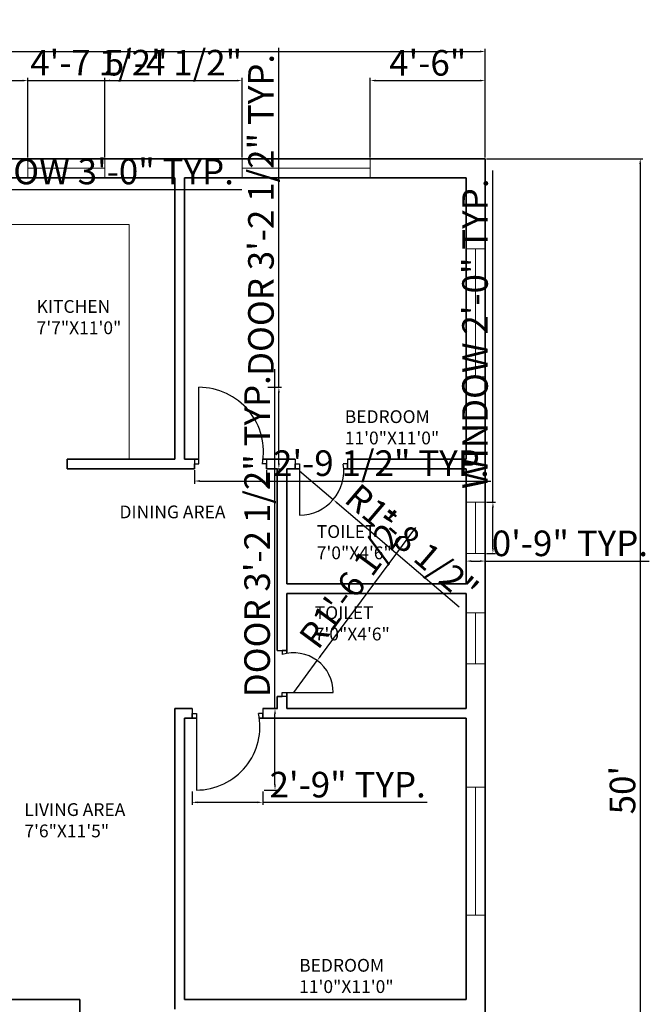
# Model space of a CAD drawing. Units: inches. Extents: x 2142 to 3604, y 1690 to 2981.
# Tile 3 of 9: x 2532 to 2827, y 2019 to 2481. Entities that reach past the tile are written whole.
import ezdxf

# ---------------------------------------------------------------- set-up
doc = ezdxf.new("R2010")
doc.units = ezdxf.units.IN
for name, color, linetype, lineweight in [('A-ANNO-DIMS', 2, 'Continuous', 18), ('A-AREA-IDEN', 7, 'Continuous', 18), ('A-DOOR', 4, 'Continuous', 25), ('A-FLOR-FIXT', 8, 'Continuous', 18), ('A-GLAZ', 4, 'Continuous', 18), ('A-WALL', 7, 'Continuous', 35)]:
    doc.layers.add(name, color=color, linetype=linetype, lineweight=lineweight)
doc.styles.get("Standard").update_dxf_attribs({"font": 'arial.ttf'})
doc.dimstyles.new('ISO-25', dxfattribs={"dimtxt": 12, "dimasz": 2.5, "dimexe": 1.25, "dimexo": 0.625, "dimtad": 1, "dimdec": 0, "dimlunit": 3, "dimtxsty": 'Standard', "dimcen": 2.5, "dimadec": 0, "dimazin": 0, "dimtfac": 1, "dimtdec": 0, "dimtmove": 0, "dimatfit": 3, "dimfxl": 1, "dimarcsym": 0})

# ---------------------------------------------------------------- blocks, each defined once
blk = doc.blocks.new('*D1')
at = {"layer": 'A-ANNO-DIMS', "color": 0, "lineweight": -2, "transparency": 16777216}
for p, q in [((2272.99, 2416.32), (2272.99, 2467.23)), ((2750.49, 2416.32), (2750.49, 2467.23)), ((2275.49, 2465.98), (2747.99, 2465.98))]:
    blk.add_line(p, q, dxfattribs=at)
at = {"layer": 'A-ANNO-DIMS', "color": 0, "transparency": 16777216}
for points in [[(2275.49, 2466.4), (2275.49, 2465.56), (2272.99, 2465.98)], [(2747.99, 2466.4), (2747.99, 2465.56), (2750.49, 2465.98)]]:
    blk.add_solid(points, dxfattribs=at)
at = {"layer": 'Defpoints', "color": 0, "transparency": 16777216}
for p in [(2750.49, 2465.98), (2272.99, 2415.7), (2750.49, 2415.7)]:
    blk.add_point(p, dxfattribs=at)
at = {"layer": 'A-ANNO-DIMS', "color": 0, "transparency": 16777216, "insert": (2511.74, 2472.73), "char_height": 12, "attachment_point": 5}
blk.add_mtext("40'", dxfattribs=at)
blk = doc.blocks.new('*D2')
at = {"layer": 'A-ANNO-DIMS', "color": 0, "lineweight": -2, "transparency": 16777216}
for p, q in [((2751.11, 2415.7), (2824.38, 2415.7)), ((2823.13, 2413.2), (2823.13, 1825.7)), ((2751.11, 1823.2), (2824.38, 1823.2))]:
    blk.add_line(p, q, dxfattribs=at)
at = {"layer": 'A-ANNO-DIMS', "color": 0, "transparency": 16777216}
for points in [[(2822.72, 2413.2), (2823.55, 2413.2), (2823.13, 2415.7)], [(2822.72, 1825.7), (2823.55, 1825.7), (2823.13, 1823.2)]]:
    blk.add_solid(points, dxfattribs=at)
at = {"layer": 'Defpoints', "color": 0, "transparency": 16777216}
for p in [(2750.49, 2415.7), (2750.49, 1823.2), (2823.13, 1823.2)]:
    blk.add_point(p, dxfattribs=at)
at = {"layer": 'A-ANNO-DIMS', "color": 0, "transparency": 16777216, "insert": (2816.38, 2119.45), "char_height": 12, "attachment_point": 5, "rotation": 90}
blk.add_mtext("50'", dxfattribs=at)
blk = doc.blocks.new('DOOR-BED-REAR-R')
for p, q in [((2, 2.25), (2, 38.25)), ((0, 4.5), (0, 0)), ((0, 0), (0, 2.25)), ((0, 2.25), (2, 2.25)), ((33.74, 2.25), (31.74, 2.25)), ((33.74, 4.5), (33.74, 0)), ((33.74, 0), (33.74, 2.25))]:
    blk.add_line(p, q)
blk.add_arc((2, 7.96), 30.29, 349.1278, 90)
blk = doc.blocks.new('DOOR-BATH-REAR-R')
for p, q in [((0, 26.25), (0, 21.75)), ((0, 21.75), (0, 24)), ((0, 24), (2, 24)), ((2, 24), (2, 0)), ((24.48, 24), (22.48, 24)), ((24.48, 26.25), (24.48, 21.75)), ((24.48, 21.75), (24.48, 24))]:
    blk.add_line(p, q)
blk.add_arc((2, 20.74), 20.74, 270, 9.0396)
blk = doc.blocks.new('DOOR-BATH-FRONT-R')
for p, q in [((0, 21.72), (4.5, 21.72)), ((4.5, 21.72), (2.25, 21.72)), ((2.25, 21.72), (2.25, 19.72)), ((4.5, 0), (0, 0)), ((0, 0), (2.25, 0)), ((2.25, 0), (2.25, 2)), ((2.25, 2), (26.25, 2))]:
    blk.add_line(p, q)
blk.add_arc((7.71, 2), 18.54, 0, 107.1246)
blk = doc.blocks.new('DOOR-BED-MID-R')
for p, q in [((0, 38.25), (0, 33.75)), ((33.13, 38.25), (33.13, 33.75)), ((0, 33.75), (0, 36)), ((0, 36), (2, 36)), ((2, 36), (2, 0)), ((33.13, 36), (31.13, 36)), ((33.13, 33.75), (33.13, 36))]:
    blk.add_line(p, q)
blk.add_arc((2, 29.79), 29.79, 270, 12.0368)
blk = doc.blocks.new('COUNTER-KITCHEN-R')
for p, q in [((0, 110.14), (69.54, 110.14)), ((69.54, 110.14), (69.54, 0))]:
    blk.add_line(p, q)
blk = doc.blocks.new('WINDOW-60')
for p, q in [((0, 60), (9, 60)), ((9, 60), (4.5, 60)), ((4.5, 60), (4.5, 0)), ((4.5, 0), (0, 0)), ((0, 0), (9, 0))]:
    blk.add_line(p, q)
blk = doc.blocks.new('WINDOW-24')
for p, q in [((0, 24), (9, 24)), ((9, 24), (4.5, 24)), ((4.5, 24), (4.5, 0)), ((4.5, 0), (0, 0)), ((0, 0), (9, 0))]:
    blk.add_line(p, q)
blk = doc.blocks.new('WINDOW-24-B')
for p, q in [((4.5, 24), (0, 24)), ((0, 24), (9, 24)), ((4.5, 0), (4.5, 24)), ((4.5, 24), (4.5, 24)), ((0, 0), (9, 0)), ((9, 0), (4.5, 0)), ((4.5, 0), (4.5, 0))]:
    blk.add_line(p, q)
blk = doc.blocks.new('WINDOW-36')
for p, q in [((0, 9), (0, 0)), ((36, 4.5), (36, 9)), ((36, 9), (36, 0)), ((0, 0), (0, 4.5)), ((0, 4.5), (36, 4.5))]:
    blk.add_line(p, q)
blk = doc.blocks.new('*D33')
at = {"layer": 'A-ANNO-DIMS', "color": 0, "lineweight": -2, "transparency": 16777216}
for p, q in [((2444.78, 2406.07), (2444.78, 2400.05)), ((2480.78, 2406.07), (2480.78, 2400.05)), ((2447.28, 2401.3), (2478.28, 2401.3)), ((2480.78, 2401.3), (2636.38, 2401.3))]:
    blk.add_line(p, q, dxfattribs=at)
at = {"layer": 'A-ANNO-DIMS', "color": 0, "transparency": 16777216}
for points in [[(2447.28, 2401.71), (2447.28, 2400.88), (2444.78, 2401.3)], [(2478.28, 2401.71), (2478.28, 2400.88), (2480.78, 2401.3)]]:
    blk.add_solid(points, dxfattribs=at)
at = {"layer": 'Defpoints', "color": 0, "transparency": 16777216}
for p in [(2444.78, 2406.7), (2480.78, 2406.7), (2480.78, 2401.3)]:
    blk.add_point(p, dxfattribs=at)
at = {"layer": 'A-ANNO-DIMS', "color": 0, "transparency": 16777216, "insert": (2559.83, 2408.13), "char_height": 12, "attachment_point": 5}
blk.add_mtext('WINDOW 3\'-0" TYP.', dxfattribs=at)
blk = doc.blocks.new('*D35')
at = {"layer": 'A-ANNO-DIMS', "color": 0, "lineweight": -2, "transparency": 16777216}
for p, q in [((2754.09, 2254.5), (2754.09, 2410.1)), ((2751.11, 2254.5), (2755.34, 2254.5)), ((2754.09, 2233), (2754.09, 2252)), ((2751.11, 2230.5), (2755.34, 2230.5))]:
    blk.add_line(p, q, dxfattribs=at)
at = {"layer": 'A-ANNO-DIMS', "color": 0, "transparency": 16777216}
for points in [[(2753.67, 2252), (2754.5, 2252), (2754.09, 2254.5)], [(2753.67, 2233), (2754.5, 2233), (2754.09, 2230.5)]]:
    blk.add_solid(points, dxfattribs=at)
at = {"layer": 'Defpoints', "color": 0, "transparency": 16777216}
for p in [(2750.49, 2254.5), (2754.09, 2254.5), (2750.49, 2230.5)]:
    blk.add_point(p, dxfattribs=at)
at = {"layer": 'A-ANNO-DIMS', "color": 0, "transparency": 16777216, "insert": (2747.25, 2333.55), "char_height": 12, "attachment_point": 5, "rotation": 90}
blk.add_mtext('WINDOW 2\'-0" TYP.', dxfattribs=at)
blk = doc.blocks.new('*D36')
at = {"layer": 'A-ANNO-DIMS', "color": 0, "lineweight": -2, "transparency": 16777216}
for p, q in [((2741.49, 2229.88), (2741.49, 2225.65)), ((2743.99, 2226.9), (2747.99, 2226.9)), ((2750.49, 2229.88), (2750.49, 2225.65)), ((2750.49, 2226.9), (2827.38, 2226.9))]:
    blk.add_line(p, q, dxfattribs=at)
at = {"layer": 'A-ANNO-DIMS', "color": 0, "transparency": 16777216}
for points in [[(2743.99, 2227.32), (2743.99, 2226.49), (2741.49, 2226.9)], [(2747.99, 2227.32), (2747.99, 2226.49), (2750.49, 2226.9)]]:
    blk.add_solid(points, dxfattribs=at)
at = {"layer": 'Defpoints', "color": 0, "transparency": 16777216}
for p in [(2741.49, 2230.5), (2750.49, 2230.5), (2750.49, 2226.9)]:
    blk.add_point(p, dxfattribs=at)
at = {"layer": 'A-ANNO-DIMS', "color": 0, "transparency": 16777216, "insert": (2790.18, 2233.66), "char_height": 12, "attachment_point": 5}
blk.add_mtext('0\'-9" TYP.', dxfattribs=at)
blk = doc.blocks.new('*D45')
at = {"layer": 'A-ANNO-DIMS', "color": 0, "lineweight": -2, "transparency": 16777216}
for p, q in [((2653.75, 2308.45), (2653.75, 2467.66)), ((2648.64, 2308.45), (2655, 2308.45)), ((2653.75, 2272.7), (2653.75, 2305.95)), ((2648.64, 2270.2), (2655, 2270.2))]:
    blk.add_line(p, q, dxfattribs=at)
at = {"layer": 'A-ANNO-DIMS', "color": 0, "transparency": 16777216}
for points in [[(2653.33, 2305.95), (2654.17, 2305.95), (2653.75, 2308.45)], [(2653.33, 2272.7), (2654.17, 2272.7), (2653.75, 2270.2)]]:
    blk.add_solid(points, dxfattribs=at)
at = {"layer": 'Defpoints', "color": 0, "transparency": 16777216}
for p in [(2648.01, 2308.45), (2653.75, 2308.45), (2648.01, 2270.2)]:
    blk.add_point(p, dxfattribs=at)
at = {"layer": 'A-ANNO-DIMS', "color": 0, "transparency": 16777216, "insert": (2646.91, 2389.3), "char_height": 12, "attachment_point": 5, "rotation": 90}
blk.add_mtext('DOOR 3\'-2 1/2" TYP.', dxfattribs=at)
blk = doc.blocks.new('*D46')
at = {"layer": 'A-ANNO-DIMS', "color": 0, "lineweight": -2, "transparency": 16777216}
for p, q in [((2614.27, 2269.57), (2614.27, 2263.21)), ((2648.01, 2269.57), (2648.01, 2263.21)), ((2616.77, 2264.46), (2645.51, 2264.46)), ((2648.01, 2264.46), (2753.07, 2264.46))]:
    blk.add_line(p, q, dxfattribs=at)
at = {"layer": 'A-ANNO-DIMS', "color": 0, "transparency": 16777216}
for points in [[(2616.77, 2264.88), (2616.77, 2264.04), (2614.27, 2264.46)], [(2645.51, 2264.88), (2645.51, 2264.04), (2648.01, 2264.46)]]:
    blk.add_solid(points, dxfattribs=at)
at = {"layer": 'Defpoints', "color": 0, "transparency": 16777216}
for p in [(2614.27, 2270.2), (2648.01, 2270.2), (2648.01, 2264.46)]:
    blk.add_point(p, dxfattribs=at)
at = {"layer": 'A-ANNO-DIMS', "color": 0, "transparency": 16777216, "insert": (2701.79, 2271.29), "char_height": 12, "attachment_point": 5}
blk.add_mtext('2\'-9 1/2" TYP.', dxfattribs=at)
blk = doc.blocks.new('*D57')
at = {"layer": 'A-ANNO-DIMS', "color": 0, "lineweight": -2, "transparency": 16777216}
for p, q in [((2651.94, 2157.7), (2651.94, 2316.91)), ((2646.83, 2157.7), (2653.19, 2157.7)), ((2651.94, 2121.95), (2651.94, 2155.2)), ((2646.83, 2119.45), (2653.19, 2119.45))]:
    blk.add_line(p, q, dxfattribs=at)
at = {"layer": 'A-ANNO-DIMS', "color": 0, "transparency": 16777216}
for points in [[(2651.53, 2155.2), (2652.36, 2155.2), (2651.94, 2157.7)], [(2651.53, 2121.95), (2652.36, 2121.95), (2651.94, 2119.45)]]:
    blk.add_solid(points, dxfattribs=at)
at = {"layer": 'Defpoints', "color": 0, "transparency": 16777216}
for p in [(2646.21, 2157.7), (2651.94, 2157.7), (2646.21, 2119.45)]:
    blk.add_point(p, dxfattribs=at)
at = {"layer": 'A-ANNO-DIMS', "color": 0, "transparency": 16777216, "insert": (2645.11, 2238.55), "char_height": 12, "attachment_point": 5, "rotation": 90}
blk.add_mtext('DOOR 3\'-2 1/2" TYP.', dxfattribs=at)
blk = doc.blocks.new('*D58')
at = {"layer": 'A-ANNO-DIMS', "color": 0, "lineweight": -2, "transparency": 16777216}
for p, q in [((2613.07, 2118.82), (2613.07, 2112.46)), ((2646.21, 2118.82), (2646.21, 2112.46)), ((2615.57, 2113.71), (2643.71, 2113.71)), ((2646.21, 2113.71), (2723.31, 2113.71))]:
    blk.add_line(p, q, dxfattribs=at)
at = {"layer": 'A-ANNO-DIMS', "color": 0, "transparency": 16777216}
for points in [[(2615.57, 2114.13), (2615.57, 2113.29), (2613.07, 2113.71)], [(2643.71, 2114.13), (2643.71, 2113.29), (2646.21, 2113.71)]]:
    blk.add_solid(points, dxfattribs=at)
at = {"layer": 'Defpoints', "color": 0, "transparency": 16777216}
for p in [(2613.07, 2119.45), (2646.21, 2119.45), (2646.21, 2113.71)]:
    blk.add_point(p, dxfattribs=at)
at = {"layer": 'A-ANNO-DIMS', "color": 0, "transparency": 16777216, "insert": (2686.01, 2120.46), "char_height": 12, "attachment_point": 5}
blk.add_mtext('2\'-9" TYP.', dxfattribs=at)
blk = doc.blocks.new('*D107')
at = {"layer": 'A-ANNO-DIMS', "color": 0, "lineweight": -2, "transparency": 16777216}
for p, q in [((2480.78, 2416.32), (2480.78, 2453.6)), ((2536.11, 2416.32), (2536.11, 2453.6)), ((2483.28, 2452.35), (2533.61, 2452.35)), ((2536.11, 2452.35), (2600.21, 2452.35))]:
    blk.add_line(p, q, dxfattribs=at)
at = {"layer": 'A-ANNO-DIMS', "color": 0, "transparency": 16777216}
for points in [[(2483.28, 2452.76), (2483.28, 2451.93), (2480.78, 2452.35)], [(2533.61, 2452.76), (2533.61, 2451.93), (2536.11, 2452.35)]]:
    blk.add_solid(points, dxfattribs=at)
at = {"layer": 'Defpoints', "color": 0, "transparency": 16777216}
for p in [(2536.11, 2452.35), (2480.78, 2415.7), (2536.11, 2415.7)]:
    blk.add_point(p, dxfattribs=at)
at = {"layer": 'A-ANNO-DIMS', "color": 0, "transparency": 16777216, "insert": (2569.41, 2459.18), "char_height": 12, "attachment_point": 5}
blk.add_mtext('4\'-7 1/2"', dxfattribs=at)
blk = doc.blocks.new('*D108')
at = {"layer": 'A-ANNO-DIMS', "color": 0, "lineweight": -2, "transparency": 16777216}
for p, q in [((2572.11, 2416.32), (2572.11, 2453.6)), ((2636.59, 2416.32), (2636.59, 2453.6)), ((2574.61, 2452.35), (2634.09, 2452.35))]:
    blk.add_line(p, q, dxfattribs=at)
at = {"layer": 'A-ANNO-DIMS', "color": 0, "transparency": 16777216}
for points in [[(2574.61, 2452.76), (2574.61, 2451.93), (2572.11, 2452.35)], [(2634.09, 2452.76), (2634.09, 2451.93), (2636.59, 2452.35)]]:
    blk.add_solid(points, dxfattribs=at)
at = {"layer": 'Defpoints', "color": 0, "transparency": 16777216}
for p in [(2636.59, 2452.35), (2572.11, 2415.7), (2636.59, 2415.7)]:
    blk.add_point(p, dxfattribs=at)
at = {"layer": 'A-ANNO-DIMS', "color": 0, "transparency": 16777216, "insert": (2604.35, 2459.18), "char_height": 12, "attachment_point": 5}
blk.add_mtext('5\'-4 1/2"', dxfattribs=at)
blk = doc.blocks.new('*D109')
at = {"layer": 'A-ANNO-DIMS', "color": 0, "lineweight": -2, "transparency": 16777216}
for p, q in [((2696.59, 2416.32), (2696.59, 2453.6)), ((2750.49, 2416.32), (2750.49, 2453.6)), ((2699.09, 2452.35), (2747.99, 2452.35))]:
    blk.add_line(p, q, dxfattribs=at)
at = {"layer": 'A-ANNO-DIMS', "color": 0, "transparency": 16777216}
for points in [[(2699.09, 2452.76), (2699.09, 2451.93), (2696.59, 2452.35)], [(2747.99, 2452.76), (2747.99, 2451.93), (2750.49, 2452.35)]]:
    blk.add_solid(points, dxfattribs=at)
at = {"layer": 'Defpoints', "color": 0, "transparency": 16777216}
for p in [(2750.49, 2452.35), (2696.59, 2415.7), (2750.49, 2415.7)]:
    blk.add_point(p, dxfattribs=at)
at = {"layer": 'A-ANNO-DIMS', "color": 0, "transparency": 16777216, "insert": (2723.54, 2459.1), "char_height": 12, "attachment_point": 5}
blk.add_mtext('4\'-6"', dxfattribs=at)
blk = doc.blocks.new('*D134')
at = {"layer": 'A-ANNO-DIMS', "color": 0, "lineweight": -2, "transparency": 16777216}
for p, q in [((2663.48, 2269.19), (2679.25, 2255.72)), ((2738.27, 2205.35), (2681.15, 2254.1))]:
    blk.add_line(p, q, dxfattribs=at)
at = {"layer": 'A-ANNO-DIMS', "color": 0, "transparency": 16777216}
blk.add_solid([(2681.42, 2254.42), (2680.88, 2253.78), (2679.25, 2255.72)], dxfattribs=at)
at = {"layer": 'Defpoints', "color": 0, "transparency": 16777216}
for p in [(2663.48, 2269.19), (2679.25, 2255.72)]:
    blk.add_point(p, dxfattribs=at)
at = {"layer": 'A-ANNO-DIMS', "color": 0, "transparency": 16777216, "insert": (2715.1, 2234.11), "char_height": 12, "attachment_point": 5, "rotation": 319.519}
blk.add_mtext('R1\'-8 1/2"', dxfattribs=at)
blk = doc.blocks.new('*D136')
at = {"layer": 'A-ANNO-DIMS', "color": 0, "lineweight": -2, "transparency": 16777216}
for p, q in [((2717.8, 2242.64), (2673.19, 2182.23)), ((2660.7, 2165.3), (2671.71, 2180.22))]:
    blk.add_line(p, q, dxfattribs=at)
at = {"layer": 'A-ANNO-DIMS', "color": 0, "transparency": 16777216}
blk.add_solid([(2672.86, 2182.48), (2673.53, 2181.98), (2671.71, 2180.22)], dxfattribs=at)
at = {"layer": 'Defpoints', "color": 0, "transparency": 16777216}
for p in [(2671.71, 2180.22), (2660.7, 2165.3)]:
    blk.add_point(p, dxfattribs=at)
at = {"layer": 'A-ANNO-DIMS', "color": 0, "transparency": 16777216, "insert": (2690.74, 2217.5), "char_height": 12, "attachment_point": 5, "rotation": 53.5617}
blk.add_mtext('R1\'-6 1/2"', dxfattribs=at)

msp = doc.modelspace()

# ---------------------------------------------------------------- linework, layer by layer
at = {"layer": 'A-WALL'}
for p, q in [((2272.99, 2415.7), (2750.49, 2415.7)), ((2272.99, 2415.7), (2750.49, 2415.7)), ((2750.49, 2415.7), (2750.49, 1823.2)), ((2513.99, 2406.7), (2604.99, 2406.7)), ((2604.99, 2406.7), (2604.99, 2274.7)), ((2609.49, 2406.7), (2609.49, 2274.7)), ((2609.49, 2406.7), (2741.49, 2406.7)), ((2741.49, 2406.7), (2741.49, 2274.7)), ((2554.48, 2274.7), (2604.99, 2274.7)), ((2554.48, 2274.7), (2554.48, 2270.2)), ((2609.49, 2274.7), (2616.27, 2274.7)), ((2646.36, 2274.7), (2661.47, 2274.7)), ((2685.96, 2274.7), (2741.49, 2274.7)), ((2554.48, 2270.2), (2614.27, 2270.2)), ((2648.01, 2270.2), (2652.99, 2270.2)), ((2652.99, 2270.2), (2652.99, 2185.02)), ((2657.49, 2216.2), (2657.49, 2270.2)), ((2657.49, 2270.2), (2663.48, 2270.2)), ((2684.19, 2270.2), (2741.49, 2270.2)), ((2741.49, 2270.2), (2741.49, 2216.2)), ((2657.49, 2216.2), (2741.49, 2216.2)), ((2657.49, 2211.7), (2741.49, 2211.7)), ((2657.49, 2183.56), (2657.49, 2211.7)), ((2741.49, 2211.7), (2741.49, 2157.7)), ((2652.99, 2163.3), (2652.99, 2157.7)), ((2657.49, 2157.7), (2657.49, 2165.3)), ((2604.99, 2157.7), (2604.99, 2016.7)), ((2604.99, 2157.7), (2604.99, 2153.2)), ((2613.07, 2157.7), (2604.99, 2157.7)), ((2652.99, 2157.7), (2646.21, 2157.7)), ((2657.49, 2157.7), (2741.49, 2157.7)), ((2609.49, 2153.2), (2609.49, 2021.2)), ((2609.49, 2153.2), (2615.07, 2153.2)), ((2644.6, 2153.2), (2652.99, 2153.2)), ((2652.99, 2153.2), (2741.49, 2153.2)), ((2741.49, 2153.2), (2657.49, 2153.2)), ((2741.49, 2153.2), (2741.49, 2021.2)), ((2560.49, 2021.2), (2513.99, 2021.2)), ((2560.49, 1884.7), (2560.49, 2021.2)), ((2741.49, 2021.2), (2609.49, 2021.2))]:
    msp.add_line(p, q, dxfattribs=at)

# ---------------------------------------------------------------- block references
at = {"layer": 'A-DOOR'}
for name, p in [('DOOR-BED-REAR-R', (2614.27, 2270.2)), ('DOOR-BATH-REAR-R', (2661.47, 2248.45)), ('DOOR-BATH-FRONT-R', (2652.99, 2163.3)), ('DOOR-BED-MID-R', (2613.07, 2119.45))]:
    msp.add_blockref(name, p, dxfattribs=at)
at = {"layer": 'A-FLOR-FIXT'}
msp.add_blockref('COUNTER-KITCHEN-R', (2513.99, 2274.7), dxfattribs=at)
at = {"layer": 'A-GLAZ'}
for name, p in [('WINDOW-36', (2536.11, 2406.7)), ('WINDOW-24-B', (2741.49, 2230.5)), ('WINDOW-24', (2741.49, 2178.63)), ('WINDOW-60', (2741.49, 2060.75))]:
    msp.add_blockref(name, p, dxfattribs=at)
at = {"layer": 'A-GLAZ', "extrusion": (0, 0, -1), "zscale": -1}
for p, rotation in [((-2696.59, 2415.7), 270), ((-2741.49, 2373.35), 180)]:
    msp.add_blockref('WINDOW-60', p, dxfattribs=dict(at, rotation=rotation))

# ---------------------------------------------------------------- texts
at = {"layer": 'A-AREA-IDEN', "char_height": 6, "attachment_point": 1}
for s, width, insert in [('KITCHEN\\P7\'7"X11\'0"', 106.5987, (2540.2, 2349.36)), ('BEDROOM\\P11\'0"X11\'0"', 75.5917, (2684.65, 2297.66)), ('DINING AREA', 86.5434, (2579.03, 2252.97)), ('TOILET\\P7\'0"X4\'6"', 54.861, (2671.51, 2243.76)), ('TOILET\\P7\'0"X4\'6"', 54.861, (2670.58, 2205.68)), ('LIVING AREA\\P7\'6"X11\'5" ', 119.5331, (2534.47, 2113.3)), ('BEDROOM\\P11\'0"X11\'0"', 121.5641, (2663.27, 2040.25))]:
    msp.add_mtext_dynamic_manual_height_columns(s, width=width, gutter_width=12.5, heights=[0], dxfattribs=dict(at, insert=insert))

# ---------------------------------------------------------------- dimensions: what is measured, and where the dimension line sits
at = {"layer": 'A-ANNO-DIMS'}
for base, p1, p2, text, override, picture, middle in [((2750.49, 2465.98), (2272.99, 2415.7), (2750.49, 2415.7), "40'", {"dimclrd": 0, "dimclre": 0, "dimclrt": 0}, '*D1', (2511.74, 2472.73)), ((2480.78, 2401.3), (2444.78, 2406.7), (2480.78, 2406.7), 'WINDOW <> TYP.', {"dimdec": 1, "dimlfac": 1, "dimrnd": 0, "dimzin": 1, "dimdsep": 46, "dimlunit": 4, "dimfrac": 2}, '*D33', (2559.83, 2408.13)), ((2648.01, 2264.46), (2614.27, 2270.2), (2648.01, 2270.2), '<> TYP.', {"dimdec": 1, "dimlfac": 1, "dimrnd": 0, "dimzin": 1, "dimdsep": 46, "dimlunit": 4, "dimfrac": 2}, '*D46', (2701.79, 2271.29)), ((2750.49, 2226.9), (2741.49, 2230.5), (2750.49, 2230.5), '<> TYP.', {"dimdec": 1, "dimlfac": 1, "dimrnd": 0, "dimzin": 1, "dimdsep": 46, "dimlunit": 4, "dimfrac": 2}, '*D36', (2790.18, 2233.66)), ((2646.21, 2113.71), (2613.07, 2119.45), (2646.21, 2119.45), '<> TYP.', {"dimdec": 1, "dimlfac": 1, "dimrnd": 0, "dimzin": 1, "dimdsep": 46, "dimlunit": 4, "dimfrac": 2}, '*D58', (2686.01, 2120.46))]:
    dim = msp.add_linear_dim(base=base, p1=p1, p2=p2, text=text, dimstyle='ISO-25', override=override, dxfattribs=at)
    dim.commit()
    dim.dimension.update_dxf_attribs({"geometry": picture, "text_midpoint": middle})
for base, p1, p2, picture, middle in [((2536.11, 2452.35), (2480.78, 2415.7), (2536.11, 2415.7), '*D107', (2569.41, 2459.18)), ((2636.59, 2452.35), (2572.11, 2415.7), (2636.59, 2415.7), '*D108', (2604.35, 2459.18)), ((2750.49, 2452.35), (2696.59, 2415.7), (2750.49, 2415.7), '*D109', (2723.54, 2459.1))]:
    dim = msp.add_linear_dim(base=base, p1=p1, p2=p2, dimstyle='ISO-25', override={"dimdec": 1, "dimlfac": 1, "dimrnd": 0, "dimzin": 1, "dimdsep": 46, "dimlunit": 4, "dimfrac": 2}, dxfattribs=at)
    dim.commit()
    dim.dimension.update_dxf_attribs({"geometry": picture, "text_midpoint": middle})
for base, p1, p2, text, override, picture, middle in [((2653.74920969, 2308.44672184), (2648.01170969, 2270.19672184), (2648.01170969, 2308.44672184), 'DOOR <> TYP.', {"dimdec": 1, "dimlfac": 1, "dimrnd": 0, "dimzin": 1, "dimdsep": 46, "dimlunit": 4, "dimfrac": 2}, '*D45', (2646.91138568, 2389.30159906)), ((2823.13, 1823.2), (2750.49, 2415.7), (2750.49, 1823.2), "50'", {"dimclrd": 0, "dimclre": 0, "dimclrt": 0}, '*D2', (2816.38, 2119.45)), ((2754.09, 2254.5), (2750.49, 2230.5), (2750.49, 2254.5), 'WINDOW <> TYP.', {"dimdec": 1, "dimlfac": 1, "dimrnd": 0, "dimzin": 1, "dimdsep": 46, "dimlunit": 4, "dimfrac": 2}, '*D35', (2747.25, 2333.55)), ((2651.94321141, 2157.69672184), (2646.20571141, 2119.44672184), (2646.20571141, 2157.69672184), 'DOOR <> TYP.', {"dimdec": 1, "dimlfac": 1, "dimrnd": 0, "dimzin": 1, "dimdsep": 46, "dimlunit": 4, "dimfrac": 2}, '*D57', (2645.1053874, 2238.55159906))]:
    dim = msp.add_linear_dim(base=base, p1=p1, p2=p2, angle=90, text=text, dimstyle='ISO-25', override=override, dxfattribs=at)
    dim.commit()
    dim.dimension.update_dxf_attribs({"geometry": picture, "text_midpoint": middle})
for center, mpoint, picture, middle in [((2663.48, 2269.19), (2679.25, 2255.72), '*D134', (2715.1, 2234.11)), ((2660.7, 2165.3), (2671.71, 2180.22), '*D136', (2690.74, 2217.5))]:
    dim = msp.add_radius_dim(center=center, mpoint=mpoint, dimstyle='ISO-25', override={"dimdec": 1, "dimlfac": 1, "dimrnd": 0, "dimzin": 1, "dimdsep": 46, "dimlunit": 4, "dimfrac": 2}, dxfattribs=at)
    dim.commit()
    dim.dimension.update_dxf_attribs({"geometry": picture, "text_midpoint": middle})

doc.saveas('drawing.dxf')
